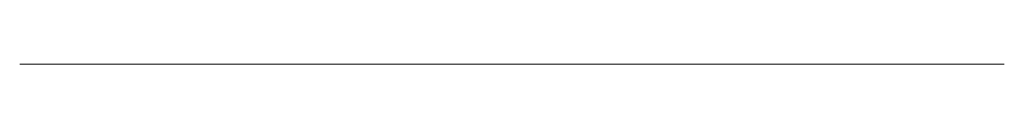
# Model space of a CAD drawing. Units: millimetres. Extents: x 475.3 to 570.3, y 0 to 0.
import ezdxf

# ---------------------------------------------------------------- set-up
doc = ezdxf.new("R2010")
doc.units = ezdxf.units.MM
doc.layers.add('M-CONS', color=8, linetype='Continuous', lineweight=18)

msp = doc.modelspace()

# ---------------------------------------------------------------- linework, layer by layer
at = {"layer": 'M-CONS', "extrusion": (0, -1, 0)}
for p, q in [((491.336, 0, 311.132), (475.336, 0, 191.132)), ((529.836, 0, 220.132), (515.836, 0, 220.132)), ((515.836, 0, 220.132), (515.836, 0, 215.132)), ((529.836, 0, 215.132), (529.836, 0, 220.132)), ((570.161, 0, 191.132), (554.336, 0, 311.132))]:
    msp.add_line(p, q, dxfattribs=at)
for centre, radius in [((522.836, 191.132), 47.5), ((522.836, 311.132), 31.5), ((522.836, 311.132), 19)]:
    msp.add_circle(centre, radius, dxfattribs=at)
msp.add_arc((522.836, 191.132), 25, 106.2602, 73.7398, dxfattribs=at)

doc.saveas('drawing.dxf')
